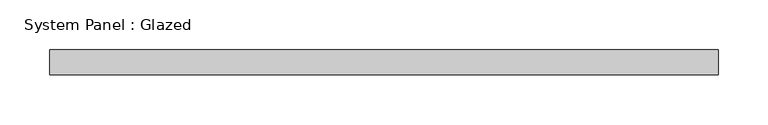
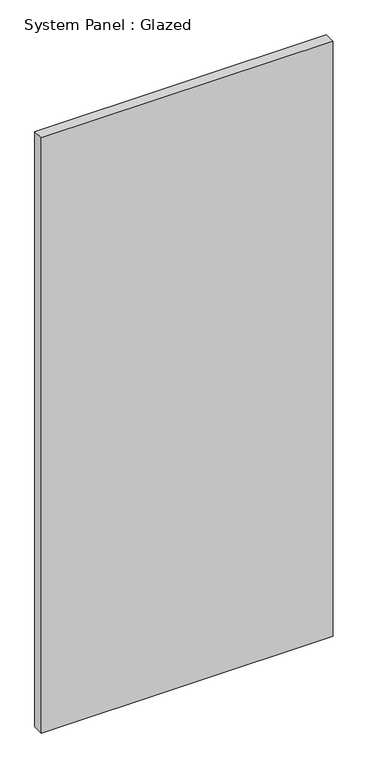
"""IFC4 building model written with IfcOpenShell, lengths in millimetres: plate geometry, System Panel : Glazed."""

from ifc_helpers import new_model, si_unit, origin, origin_with_axes, place, context, project, spatial, polyline, outline, extrude, source, transform, mapped, element, save


def system_panel_glazed_27fbb1ef(model_context):
    return source(origin(), model_context, "Body", "SweptSolid", [
        extrude(outline(polyline([(336.55, 19.05), (-336.55, 19.05), (-336.55, 44.45), (336.55, 44.45), (336.55, 19.05)])), origin_with_axes(), (0.0, 0.0, 1.0), 1451.2793787),
    ])


if __name__ == "__main__":
    model = new_model("IFC4")
    model_context = context("Model", 3, world=origin())
    ifc_project = project(units=[si_unit("LENGTHUNIT", "METRE", prefix="MILLI")], contexts=[model_context])
    site = spatial("IfcSite", under=ifc_project)
    building = spatial("IfcBuilding", under=site)
    placement = place(None, origin())
    system_panel_glazed_shape = system_panel_glazed_27fbb1ef(model_context)
    element("IfcPlate", 1, ObjectType="System Panel : Glazed", at=placement, inside=building, context=model_context, shape_type="MappedRepresentation", body=[
        mapped(system_panel_glazed_shape, transform((0.0, 0.0, 0.0), x_axis=(1.0, 0.0, 0.0), y_axis=(0.0, 1.0, 0.0), z_axis=(0.0, 0.0, 1.0))),
    ])
    save(model, "model.ifc")

# Revit data of these elements
# Type "System Panel : Glazed"
#   Construction Type Id = "GSP4R"
#   Analytic Construction = "1/8 in Pilkington single glazing"
#   Visual Light Transmittance = 0.9
#   Solar Heat Gain Coefficient = 0.86
#   Heat Transfer Coefficient (U) = 1.18115 BTU/(h·ft²·°F)
#   Define Thermal Properties by = 1
# Element 1 (IfcPlate, "System Panel : Glazed")
#   Materials on its faces: "Glass"
# Materials
#   "Glass": class "Glass", colour RGB 0 128 192, transparency 0.75, Description = "Soda Lime Glass", Cost = 0
